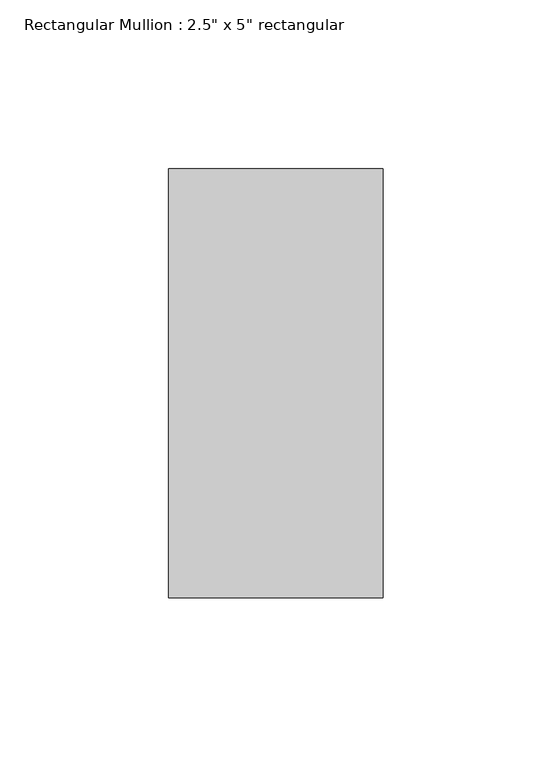
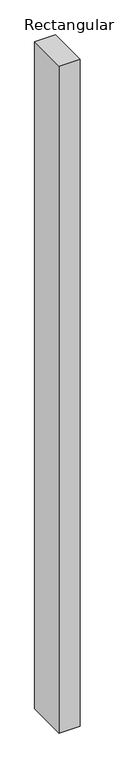
"""IFC4 building model written with IfcOpenShell, lengths in millimetres: member geometry."""

from ifc_helpers import new_model, si_unit, frame, origin, place, context, project, spatial, polyline, outline, extrude, source, transform, mapped, element, save


def member_3a4673bc(model_context):
    return source(origin(), model_context, "Body", "SweptSolid", [
        extrude(outline(polyline([(0.0, 63.5), (0.0, -63.5), (-63.5, -63.5), (-63.5, 63.5), (0.0, 63.5)])), frame((0.0, 0.0, -2128.2825), z_axis=(0.0, 0.0, 1.0), x_axis=(1.0, 0.0, 0.0)), (0.0, 0.0, 1.0), 2128.2825),
    ])


if __name__ == "__main__":
    model = new_model("IFC4")
    model_context = context("Model", 3, world=origin())
    ifc_project = project(units=[si_unit("LENGTHUNIT", "METRE", prefix="MILLI")], contexts=[model_context])
    site = spatial("IfcSite", under=ifc_project)
    building = spatial("IfcBuilding", under=site)
    placement = place(None, origin())
    member_shape = member_3a4673bc(model_context)
    element("IfcMember", 1, ObjectType="Rectangular Mullion : 2.5\" x 5\" rectangular", at=placement, inside=building, context=model_context, shape_type="MappedRepresentation", body=[
        mapped(member_shape, transform((0.0, 0.0, 0.0), x_axis=(1.0, 0.0, 0.0), y_axis=(0.0, 1.0, 0.0), z_axis=(0.0, 0.0, 1.0))),
    ])
    save(model, "model.ifc")

# Revit data of these elements
# Type "Rectangular Mullion : 2.5\" x 5\" rectangular"
#   built-in parameter 1007304 = 0.416667 (stored number, unit not read)
#   built-in parameter 1007301 = 0.104167 (stored number, unit not read)
#   built-in parameter 1007300 = 0.104167 (stored number, unit not read)
# Element 1 (IfcMember, "Rectangular Mullion : 2.5\" x 5\" rectangular")
#   Materials on its faces: "Aluminum"
# Materials
#   "Aluminum": class "Metal", colour RGB 247 247 247, transparency 0, Description = "Aluminum 6061", Cost = 0
